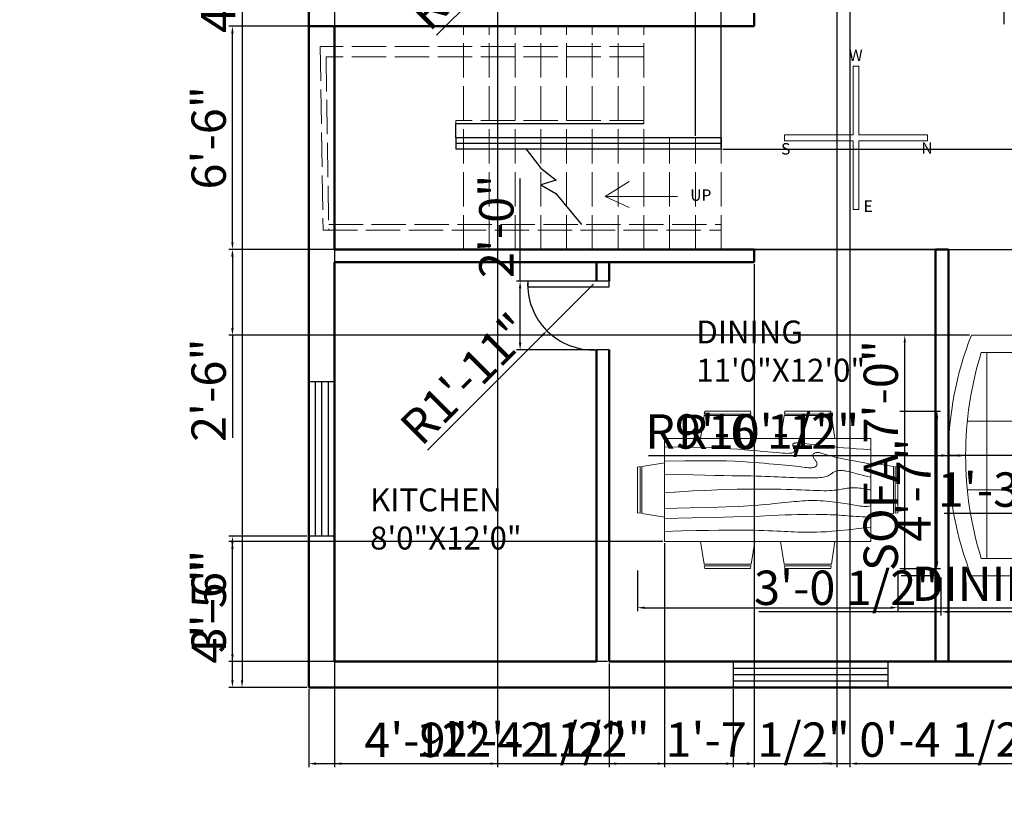
# Model space of a CAD drawing. Units: inches. Extents: x 2787 to 3354, y 1541 to 2259.
# Tile 1 of 3: x 2787 to 3131, y 1571 to 1842. Entities that reach past the tile are written whole.
import ezdxf

# ---------------------------------------------------------------- set-up
doc = ezdxf.new("R2010")
doc.units = ezdxf.units.IN
doc.linetypes.add('ACAD_ISO02W100', pattern=[15, 12, -3])
for name, color, linetype, lineweight in [('A-ANNO-DIMS', 2, 'Continuous', 18), ('A-ANNO-SYMB', 7, 'Continuous', 18), ('A-ANNO-TEXT', 7, 'Continuous', 18), ('A-AREA-IDEN', 7, 'Continuous', 25), ('A-DOOR', 4, 'Continuous', 25), ('A-FLOR-STRS', 7, 'Continuous', 25), ('A-FLOR-STRS-OVHD', 7, 'ACAD_ISO02W100', 18), ('A-FURN', 8, 'Continuous', 18), ('A-GLAZ', 4, 'Continuous', 25), ('A-WALL', 7, 'Continuous', 50)]:
    doc.layers.add(name, color=color, linetype=linetype, lineweight=lineweight)
doc.styles.get("Standard").update_dxf_attribs({"font": 'arial.ttf'})
doc.dimstyles.new('ISO-25', dxfattribs={"dimtxt": 12, "dimasz": 2.5, "dimexe": 1.25, "dimexo": 0.625, "dimtad": 1, "dimdec": 1, "dimlunit": 3, "dimtxsty": 'Standard', "dimcen": 2.5, "dimadec": 0, "dimazin": 0, "dimtfac": 1, "dimtdec": 1, "dimtmove": 0, "dimatfit": 3, "dimfxl": 1, "dimarcsym": 0})

# ---------------------------------------------------------------- blocks, each defined once
blk = doc.blocks.new('Window - Wood Frame 36 in. Wide plan')
for p, q in [((0, 6), (0, 0)), ((36, 6), (36, 0)), ((0, 4.5), (36, 4.5)), ((0, 3), (36, 3)), ((0, 1.5), (36, 1.5))]:
    blk.add_line(p, q)
blk = doc.blocks.new('Dining Set - 36 x 72 in.')
for p, q in [((-22.2343, 26.00059), (-23.4847, 17.99762)), ((-22.2304, 26), (-5.7608, 26)), ((-22, 27.5), (-22.1562, 26.50042)), ((-5.8416, 26.5), (-22.1534, 26.5)), ((-22, 27.5), (-6, 27.5)), ((-5.8437, 26.49966), (-6, 27.5)), ((-4.5152, 17.99762), (-5.7655, 25.99926)), ((5.7657, 26.00059), (4.5153, 17.99762)), ((5.7696, 26), (22.2392, 26)), ((6, 27.5), (5.8438, 26.50042)), ((22.1584, 26.5), (5.8466, 26.5)), ((6, 27.5), (22, 27.5)), ((22.1563, 26.49966), (22, 27.5)), ((23.4848, 17.99762), (22.2345, 25.99926)), ((36, 18), (-36, 18)), ((-36, 18), (-36, -18)), ((36, -18), (36, 18)), ((-45.5, 8), (-44.5004, 8.15617)), ((-45.5, 8), (-45.5, -8)), ((-44.5, -8.15843), (-44.5, 8.15338)), ((-44.0006, 8.23428), (-35.9976, 9.48474)), ((-44, 8.23041), (-44, -8.23915)), ((44.0006, 8.23428), (35.9976, 9.48474)), ((44, 8.23041), (44, -8.23915)), ((44.5, -8.15843), (44.5, 8.15338)), ((45.5, 8), (44.5005, 8.15617)), ((45.5, 8), (45.5, -8)), ((-44.4997, -8.15631), (-45.5, -8)), ((-35.9976, -9.48476), (-43.9993, -8.2345)), ((35.9976, -9.48476), (43.9993, -8.2345)), ((44.4997, -8.15631), (45.5, -8)), ((-36, -18), (36, -18)), ((-22.2343, -26.0006), (-23.4847, -17.99762)), ((-4.5152, -17.99762), (-5.7655, -25.99928)), ((5.7657, -26.0006), (4.5153, -17.99762)), ((23.4848, -17.99762), (22.2345, -25.99928)), ((-22.2304, -26), (-5.7608, -26)), ((-22, -27.5), (-22.1562, -26.50044)), ((-5.8416, -26.5), (-22.1534, -26.5)), ((-22, -27.5), (-6, -27.5)), ((-5.8437, -26.49967), (-6, -27.5)), ((5.7696, -26), (22.2392, -26)), ((6, -27.5), (5.8438, -26.50044)), ((22.1584, -26.5), (5.8466, -26.5)), ((6, -27.5), (22, -27.5)), ((22.1563, -26.49967), (22, -27.5))]:
    blk.add_line(p, q)
for points in [[(-36, 15), (-31.1772, 14.97754), (-26.8079, 14.91406), (-22.8538, 14.81543), (-19.276, 14.6875), (-16.0362, 14.53613), (-13.0957, 14.36718), (-10.4159, 14.18652), (-7.9583, 14), (-5.6904, 13.81315), (-3.6035, 13.63021), (-1.6954, 13.45508), (0.0365, 13.29166), (1.5945, 13.14388), (2.9811, 13.01562), (4.1988, 12.9108), (5.25, 12.83333), (6.1393, 12.78613), (6.8802, 12.76823), (7.4883, 12.77767), (7.9792, 12.8125), (8.3685, 12.87077), (8.6719, 12.95052), (8.9049, 13.0498), (9.0833, 13.16666), (9.2205, 13.29899), (9.3216, 13.44401), (9.3895, 13.59879), (9.4271, 13.76041), (9.4373, 13.92594), (9.4232, 14.09245), (9.3875, 14.257), (9.3333, 14.41666), (9.2638, 14.56917), (9.1836, 14.71484), (9.0975, 14.85465), (9.0104, 14.98958), (8.9272, 15.1206), (8.8529, 15.2487), (8.7922, 15.37483), (8.75, 15.5), (8.7305, 15.62467), (8.7344, 15.74739), (8.7617, 15.86621), (8.8125, 15.97916), (8.8867, 16.08431), (8.9844, 16.17968), (9.1055, 16.26334), (9.25, 16.33333), (9.4189, 16.38802), (9.6172, 16.42708), (9.8506, 16.45052), (10.125, 16.45833), (10.4463, 16.45052), (10.8203, 16.42708), (11.2529, 16.38802), (11.75, 16.33333), (12.3184, 16.26318), (12.9694, 16.17838), (13.7151, 16.07991), (14.5677, 15.96875), (15.5395, 15.84586), (16.6426, 15.71224), (17.8893, 15.56884), (19.2917, 15.41666), (20.859, 15.25667), (22.5879, 15.08984), (24.4721, 14.91715), (26.5052, 14.73958), (28.6809, 14.5581), (30.9929, 14.3737), (33.4347, 14.18733), (36, 14)], [(-36, 10), (-28.9766, 10.14274), (-23.1725, 10.20442), (-18.4241, 10.19775), (-14.5677, 10.13541), (-11.4399, 10.03011), (-8.877, 9.89453), (-6.7154, 9.74137), (-4.7917, 9.58333), (-2.9698, 9.43082), (-1.2246, 9.28515), (0.4415, 9.14534), (2.026, 9.01041), (3.5266, 8.87939), (4.9408, 8.7513), (6.266, 8.62516), (7.5, 8.5), (8.6411, 8.37549), (9.6914, 8.2539), (10.6538, 8.13818), (11.5312, 8.03125), (12.3267, 7.93603), (13.043, 7.85547), (13.6831, 7.79248), (14.25, 7.75), (14.7471, 7.7303), (15.1797, 7.73307), (15.5537, 7.75732), (15.875, 7.80208), (16.1494, 7.86637), (16.3828, 7.94922), (16.5811, 8.04964), (16.75, 8.16666), (16.8944, 8.29915), (17.0143, 8.44531), (17.1089, 8.60319), (17.1771, 8.77083), (17.218, 8.94629), (17.2305, 9.1276), (17.2137, 9.31282), (17.1667, 9.5), (17.0895, 9.6875), (16.987, 9.875), (16.8649, 10.0625), (16.7292, 10.25), (16.5856, 10.4375), (16.4401, 10.625), (16.2985, 10.8125), (16.1667, 11), (16.05, 11.18733), (15.9518, 11.3737), (15.8752, 11.5581), (15.8229, 11.73958), (15.798, 11.91715), (15.8034, 12.08984), (15.842, 12.25667), (15.9167, 12.41666), (16.0295, 12.56836), (16.1784, 12.70833), (16.3605, 12.83268), (16.5729, 12.9375), (16.8127, 13.01888), (17.0768, 13.07291), (17.3625, 13.0957), (17.6667, 13.08333), (17.9894, 13.03312), (18.3418, 12.94726), (18.7382, 12.82918), (19.1927, 12.68229), (19.7195, 12.51001), (20.3327, 12.31575), (21.0465, 12.10294), (21.875, 11.875), (22.8357, 11.63354), (23.959, 11.37304), (25.2786, 11.08618), (26.8282, 10.76562), (28.6414, 10.40405), (30.752, 9.99414), (33.1936, 9.52856), (36, 9)], [(-36, 5.5), (-30.7157, 5.3348), (-26.069, 5.20963), (-21.9946, 5.11767), (-18.4271, 5.05208), (-15.3009, 5.00602), (-12.5508, 4.97265), (-10.1112, 4.94515), (-7.9167, 4.91666), (-5.909, 4.88167), (-4.0586, 4.83984), (-2.3429, 4.79215), (-0.7396, 4.73958), (0.7739, 4.6831), (2.22, 4.6237), (3.6213, 4.56233), (5, 4.5), (6.373, 4.43782), (7.7344, 4.3776), (9.0723, 4.32129), (10.375, 4.27083), (11.6309, 4.22819), (12.8281, 4.19531), (13.9551, 4.17415), (15, 4.16666), (15.954, 4.17448), (16.819, 4.19791), (17.6001, 4.23698), (18.3021, 4.29166), (18.9299, 4.36198), (19.4883, 4.44791), (19.9823, 4.54948), (20.4167, 4.66666), (20.7969, 4.79899), (21.1302, 4.94401), (21.4245, 5.09879), (21.6875, 5.26041), (21.9271, 5.42594), (22.1511, 5.59245), (22.3672, 5.757), (22.5834, 5.91666), (22.8065, 6.06868), (23.0404, 6.21093), (23.2879, 6.34147), (23.5521, 6.45833), (23.8358, 6.55957), (24.142, 6.64323), (24.4735, 6.70735), (24.8334, 6.75), (25.2235, 6.76969), (25.642, 6.76692), (26.0858, 6.74267), (26.5521, 6.69791), (27.0379, 6.63362), (27.5404, 6.55078), (28.0565, 6.45036), (28.5834, 6.33333), (29.1242, 6.19987), (29.7071, 6.04687), (30.3661, 5.87044), (31.1354, 5.66666), (32.0493, 5.43164), (33.142, 5.16146), (34.4475, 4.85221), (36, 4.5)], [(-36, -1), (-30.7915, -0.6591), (-26.0195, -0.38216), (-21.6519, -0.16284), (-17.6563, 0.00521), (-14.0005, 0.12833), (-10.6523, 0.21289), (-7.5796, 0.26522), (-4.75, 0.29166), (-2.134, 0.29793), (0.2878, 0.28711), (2.5317, 0.26163), (4.6146, 0.22396), (6.5529, 0.17651), (8.3633, 0.12174), (10.0623, 0.06209), (11.6667, 0), (13.1899, -0.06201), (14.6341, -0.1211), (15.9982, -0.17432), (17.2813, -0.21875), (18.4823, -0.25147), (19.6003, -0.26953), (20.6343, -0.27002), (21.5834, -0.25), (22.4481, -0.20768), (23.2357, -0.14584), (23.9549, -0.06836), (24.6146, 0.02083), (25.2235, 0.11784), (25.7904, 0.21875), (26.3241, 0.31966), (26.8334, 0.41666), (27.3265, 0.50618), (27.8099, 0.58593), (28.2894, 0.65397), (28.7709, 0.70833), (29.2601, 0.74707), (29.763, 0.76823), (30.2855, 0.76985), (30.8334, 0.75), (31.4088, 0.70784), (31.9994, 0.64713), (32.589, 0.57275), (33.1615, 0.48958), (33.7008, 0.4025), (34.1908, 0.3164), (34.6153, 0.23616), (34.9584, 0.16666), (35.2099, 0.11165), (35.3848, 0.07031), (35.504, 0.04069), (35.5886, 0.02083), (35.6594, 0.00879), (35.7377, 0.0026), (35.8442, 0.00032), (36, 0)], [(-36, -6.5), (-27.1843, -6.31267), (-20.084, -6.1263), (-14.469, -5.9419), (-10.1094, -5.76042), (-6.7752, -5.58285), (-4.2363, -5.41016), (-2.2629, -5.24333), (-0.625, -5.08334), (0.8708, -4.93099), (2.2715, -4.78646), (3.5872, -4.64974), (4.8281, -4.52084), (6.0046, -4.39974), (7.127, -4.28646), (8.2053, -4.18099), (9.25, -4.08334), (10.2705, -3.99382), (11.2734, -3.91407), (12.2647, -3.84603), (13.25, -3.79167), (14.2354, -3.75293), (15.2266, -3.73177), (16.2295, -3.73015), (17.25, -3.75), (18.2912, -3.79248), (19.3451, -3.85547), (20.4009, -3.93604), (21.4479, -4.03125), (22.4754, -4.13819), (23.4727, -4.25391), (24.4289, -4.37549), (25.3334, -4.5), (26.1785, -4.62492), (26.9694, -4.74935), (27.7145, -4.87281), (28.4219, -4.99479), (29.1, -5.11483), (29.7572, -5.23242), (30.4016, -5.34709), (31.0417, -5.45834), (31.6837, -5.56437), (32.3262, -5.65821), (32.9658, -5.73153), (33.599, -5.77604), (34.2224, -5.78345), (34.8327, -5.74545), (35.4264, -5.65373), (36, -5.5)], [(-36, -10), (-26.4022, -9.81299), (-18.4675, -9.62891), (-11.9839, -9.45069), (-6.7396, -9.28125), (-2.5226, -9.12354), (0.8789, -8.98047), (3.6769, -8.85498), (6.0833, -8.75), (8.2767, -8.66765), (10.3021, -8.60677), (12.1712, -8.56543), (13.8958, -8.54167), (15.4876, -8.53353), (16.9583, -8.53907), (18.3197, -8.55632), (19.5834, -8.58334), (20.7616, -8.61841), (21.8685, -8.66081), (22.9188, -8.71004), (23.9271, -8.76563), (24.9081, -8.82707), (25.8763, -8.89388), (26.8465, -8.96558), (27.8334, -9.04167), (28.8474, -9.12118), (29.8828, -9.20117), (30.93, -9.27824), (31.9792, -9.34896), (33.0205, -9.40991), (34.0443, -9.45768), (35.0407, -9.48885), (36, -9.5)], [(-36, -14.5), (-30.0881, -14.33513), (-25.0332, -14.21224), (-20.7312, -14.12647), (-17.0781, -14.07292), (-13.97, -14.04671), (-11.3027, -14.04297), (-8.9724, -14.05681), (-6.875, -14.08334), (-4.9224, -14.11833), (-3.0905, -14.16016), (-1.3709, -14.20785), (0.2448, -14.26042), (1.7647, -14.3169), (3.1973, -14.3763), (4.5507, -14.43767), (5.8333, -14.5), (7.0554, -14.5621), (8.235, -14.62175), (9.3922, -14.67652), (10.5469, -14.72396), (11.7192, -14.76164), (12.929, -14.78711), (14.1965, -14.79794), (15.5417, -14.79167), (16.9933, -14.76424), (18.6152, -14.70508), (20.4804, -14.60197), (22.6615, -14.44271), (25.2312, -14.21509), (28.2624, -13.9069), (31.8277, -13.50594), (36, -13)]]:
    blk.add_lwpolyline(points)
blk = doc.blocks.new('*D6')
at = {"layer": 'A-ANNO-DIMS', "color": 0, "lineweight": -2, "transparency": 16777216}
for p, q in [((2887.4, 2088.26), (2863.48, 2088.26)), ((2864.73, 2085.76), (2864.73, 1610.76)), ((2887.4, 1608.26), (2863.48, 1608.26))]:
    blk.add_line(p, q, dxfattribs=at)
at = {"layer": 'A-ANNO-DIMS', "color": 0, "transparency": 16777216}
for points in [[(2864.31, 2085.76), (2865.14, 2085.76), (2864.73, 2088.26)], [(2864.31, 1610.76), (2865.14, 1610.76), (2864.73, 1608.26)]]:
    blk.add_solid(points, dxfattribs=at)
at = {"layer": 'Defpoints', "color": 0, "transparency": 16777216}
for p in [(2888.02, 2088.26), (2864.73, 1608.26), (2888.02, 1608.26)]:
    blk.add_point(p, dxfattribs=at)
at = {"layer": 'A-ANNO-DIMS', "color": 0, "transparency": 16777216, "insert": (2857.97, 1848.26), "char_height": 12, "attachment_point": 5, "rotation": 90}
blk.add_mtext("40'", dxfattribs=at)
blk = doc.blocks.new('Sofa - Roundback 7 ft.')
for p, q in [((-12.00002, -32.4421), (-12.00003, -6.5971)), ((11.99997, -32.4421), (11.99998, -6.5971)), ((-36.000027, -34), (-36.000027, -11.4696)), ((-35.999844, -13.3819), (35.9998, -13.3819)), ((35.99998, -34), (35.99998, -11.4696)), ((-36.000027, -32.4421), (35.99998, -32.4421))]:
    blk.add_line(p, q)
for points in [[(-36.000027, -34), (-42.000027, -34), (-42.000027, -8)], [(41.99998, -8), (41.99998, -34), (35.99998, -34)]]:
    blk.add_lwpolyline(points)
for centre, radius, start, end in [((0, -114.25), 114.25, 68.43141, 111.5686), ((-0.00001, -127.1968), 121.1968, 72.72033, 107.2797)]:
    blk.add_arc(centre, radius, start, end)
blk = doc.blocks.new('*D18')
at = {"layer": 'A-ANNO-DIMS', "color": 0, "lineweight": -2, "transparency": 16777216}
for p, q in [((2897.02, 1864.37), (2897.02, 1858.79)), ((2930.07, 1864.37), (2930.07, 1858.79)), ((2897.02, 1860.04), (2787.05, 1860.04)), ((2927.57, 1860.04), (2899.52, 1860.04))]:
    blk.add_line(p, q, dxfattribs=at)
at = {"layer": 'A-ANNO-DIMS', "color": 0, "transparency": 16777216}
for points in [[(2899.52, 1860.45), (2899.52, 1859.62), (2897.02, 1860.04)], [(2927.57, 1860.45), (2927.57, 1859.62), (2930.07, 1860.04)]]:
    blk.add_solid(points, dxfattribs=at)
at = {"layer": 'Defpoints', "color": 0, "transparency": 16777216}
for p in [(2897.02, 1864.99), (2930.07, 1864.99), (2897.02, 1860.04)]:
    blk.add_point(p, dxfattribs=at)
at = {"layer": 'A-ANNO-DIMS', "color": 0, "transparency": 16777216, "insert": (2840.79, 1866.87), "char_height": 12, "attachment_point": 5}
blk.add_mtext('WC 2\'-9" TYP.', dxfattribs=at)
blk = doc.blocks.new('*D24')
at = {"layer": 'A-ANNO-DIMS', "color": 0, "lineweight": -2, "transparency": 16777216}
for p, q in [((3002.87, 1649.12), (3002.87, 1634.84)), ((3093.87, 1649.12), (3093.87, 1634.84)), ((3005.37, 1636.09), (3091.37, 1636.09)), ((3093.87, 1636.09), (3229.51, 1636.09))]:
    blk.add_line(p, q, dxfattribs=at)
at = {"layer": 'A-ANNO-DIMS', "color": 0, "transparency": 16777216}
for points in [[(3005.37, 1636.51), (3005.37, 1635.68), (3002.87, 1636.09)], [(3091.37, 1636.51), (3091.37, 1635.68), (3093.87, 1636.09)]]:
    blk.add_solid(points, dxfattribs=at)
at = {"layer": 'Defpoints', "color": 0, "transparency": 16777216}
for p in [(3002.87, 1649.74), (3093.87, 1649.74), (3093.87, 1636.09)]:
    blk.add_point(p, dxfattribs=at)
at = {"layer": 'A-ANNO-DIMS', "color": 0, "transparency": 16777216, "insert": (3162.94, 1642.92), "char_height": 12, "attachment_point": 5}
blk.add_mtext('DINING SET 7\'-7"', dxfattribs=at)
blk = doc.blocks.new('*D25')
at = {"layer": 'A-ANNO-DIMS', "color": 0, "lineweight": -2, "transparency": 16777216}
for p, q in [((3094.49, 1704.74), (3108.77, 1704.74)), ((3107.52, 1652.24), (3107.52, 1702.24)), ((3094.49, 1649.74), (3108.77, 1649.74))]:
    blk.add_line(p, q, dxfattribs=at)
at = {"layer": 'A-ANNO-DIMS', "color": 0, "transparency": 16777216}
for points in [[(3107.1, 1702.24), (3107.94, 1702.24), (3107.52, 1704.74)], [(3107.1, 1652.24), (3107.94, 1652.24), (3107.52, 1649.74)]]:
    blk.add_solid(points, dxfattribs=at)
at = {"layer": 'Defpoints', "color": 0, "transparency": 16777216}
for p in [(3093.87, 1704.74), (3107.52, 1704.74), (3093.87, 1649.74)]:
    blk.add_point(p, dxfattribs=at)
at = {"layer": 'A-ANNO-DIMS', "color": 0, "transparency": 16777216, "insert": (3100.89, 1677.24), "char_height": 12, "attachment_point": 5, "rotation": 90}
blk.add_mtext('4\'-7"', dxfattribs=at)
blk = doc.blocks.new('*D26')
at = {"layer": 'A-ANNO-DIMS', "color": 0, "lineweight": -2, "transparency": 16777216}
for p, q in [((3108.23, 1731.26), (3095.01, 1731.26)), ((3096.26, 1649.76), (3096.26, 1728.76)), ((3108.23, 1647.26), (3095.01, 1647.26))]:
    blk.add_line(p, q, dxfattribs=at)
at = {"layer": 'A-ANNO-DIMS', "color": 0, "transparency": 16777216}
for points in [[(3095.84, 1728.76), (3096.67, 1728.76), (3096.26, 1731.26)], [(3095.84, 1649.76), (3096.67, 1649.76), (3096.26, 1647.26)]]:
    blk.add_solid(points, dxfattribs=at)
at = {"layer": 'Defpoints', "color": 0, "transparency": 16777216}
for p in [(3096.26, 1731.26), (3108.86, 1731.26), (3108.86, 1647.26)]:
    blk.add_point(p, dxfattribs=at)
at = {"layer": 'A-ANNO-DIMS', "color": 0, "transparency": 16777216, "insert": (3089.42, 1689.26), "char_height": 12, "attachment_point": 5, "rotation": 90}
blk.add_mtext('SOFA 7\'-0"', dxfattribs=at)
blk = doc.blocks.new('*D27')
at = {"layer": 'A-ANNO-DIMS', "color": 0, "lineweight": -2, "transparency": 16777216}
for p, q in [((3108.86, 1646.64), (3108.86, 1633.41)), ((3145.52, 1646.64), (3145.52, 1633.41)), ((3108.86, 1634.66), (3045.25, 1634.66)), ((3143.02, 1634.66), (3111.36, 1634.66))]:
    blk.add_line(p, q, dxfattribs=at)
at = {"layer": 'A-ANNO-DIMS', "color": 0, "transparency": 16777216}
for points in [[(3111.36, 1635.08), (3111.36, 1634.24), (3108.86, 1634.66)], [(3143.02, 1635.08), (3143.02, 1634.24), (3145.52, 1634.66)]]:
    blk.add_solid(points, dxfattribs=at)
at = {"layer": 'Defpoints', "color": 0, "transparency": 16777216}
for p in [(3108.86, 1647.26), (3145.52, 1647.26), (3108.86, 1634.66)]:
    blk.add_point(p, dxfattribs=at)
at = {"layer": 'A-ANNO-DIMS', "color": 0, "transparency": 16777216, "insert": (3075.81, 1641.49), "char_height": 12, "attachment_point": 5}
blk.add_mtext('3\'-0 1/2"', dxfattribs=at)
blk = doc.blocks.new('*D31')
at = {"layer": 'A-ANNO-DIMS', "color": 0, "lineweight": -2, "transparency": 16777216}
for p, q in [((3172.5, 1672.84), (3172.5, 1667.72)), ((3188, 1672.84), (3188, 1667.72)), ((3172.5, 1668.97), (3110.02, 1668.97)), ((3185.5, 1668.97), (3175, 1668.97))]:
    blk.add_line(p, q, dxfattribs=at)
at = {"layer": 'A-ANNO-DIMS', "color": 0, "transparency": 16777216}
for points in [[(3175, 1669.39), (3175, 1668.55), (3172.5, 1668.97)], [(3185.5, 1669.39), (3185.5, 1668.55), (3188, 1668.97)]]:
    blk.add_solid(points, dxfattribs=at)
at = {"layer": 'Defpoints', "color": 0, "transparency": 16777216}
for p in [(3172.5, 1673.47), (3188, 1673.47), (3172.5, 1668.97)]:
    blk.add_point(p, dxfattribs=at)
at = {"layer": 'A-ANNO-DIMS', "color": 0, "transparency": 16777216, "insert": (3140.01, 1675.8), "char_height": 12, "attachment_point": 5}
blk.add_mtext('1\'-3 1/2"', dxfattribs=at)
blk = doc.blocks.new('*D36')
at = {"layer": 'A-ANNO-DIMS', "color": 0, "lineweight": -2, "transparency": 16777216}
for p, q in [((2887.4, 1661.04), (2860.12, 1661.04)), ((2861.37, 1610.76), (2861.37, 1658.54)), ((2887.4, 1608.26), (2860.12, 1608.26))]:
    blk.add_line(p, q, dxfattribs=at)
at = {"layer": 'A-ANNO-DIMS', "color": 0, "transparency": 16777216}
for points in [[(2860.96, 1658.54), (2861.79, 1658.54), (2861.37, 1661.04)], [(2860.96, 1610.76), (2861.79, 1610.76), (2861.37, 1608.26)]]:
    blk.add_solid(points, dxfattribs=at)
at = {"layer": 'Defpoints', "color": 0, "transparency": 16777216}
for p in [(2861.37, 1661.04), (2888.02, 1661.04), (2888.02, 1608.26)]:
    blk.add_point(p, dxfattribs=at)
at = {"layer": 'A-ANNO-DIMS', "color": 0, "transparency": 16777216, "insert": (2854.65, 1634.65), "char_height": 12, "attachment_point": 5, "rotation": 90}
blk.add_mtext('4\'-5"', dxfattribs=at)
blk = doc.blocks.new('*D40')
at = {"layer": 'A-ANNO-DIMS', "color": 0, "lineweight": -2, "transparency": 16777216}
for p, q in [((2888.02, 1607.64), (2888.02, 1580.36)), ((3036.32, 1607.64), (3036.32, 1580.36)), ((2890.52, 1581.61), (3033.82, 1581.61))]:
    blk.add_line(p, q, dxfattribs=at)
at = {"layer": 'A-ANNO-DIMS', "color": 0, "transparency": 16777216}
for points in [[(2890.52, 1582.03), (2890.52, 1581.19), (2888.02, 1581.61)], [(3033.82, 1582.03), (3033.82, 1581.19), (3036.32, 1581.61)]]:
    blk.add_solid(points, dxfattribs=at)
at = {"layer": 'Defpoints', "color": 0, "transparency": 16777216}
for p in [(2888.02, 1608.26), (3036.32, 1608.26), (3036.32, 1581.61)]:
    blk.add_point(p, dxfattribs=at)
at = {"layer": 'A-ANNO-DIMS', "color": 0, "transparency": 16777216, "insert": (2962.17, 1588.44), "char_height": 12, "attachment_point": 5}
blk.add_mtext('12\'-4 1/2"', dxfattribs=at)
blk = doc.blocks.new('*D43')
at = {"layer": 'A-ANNO-DIMS', "color": 0, "lineweight": -2, "transparency": 16777216}
for p, q in [((2961.87, 1750.14), (2961.87, 1785.99)), ((2987.9, 1750.14), (2960.62, 1750.14)), ((2961.87, 1728.64), (2961.87, 1747.64)), ((2987.9, 1726.14), (2960.62, 1726.14))]:
    blk.add_line(p, q, dxfattribs=at)
at = {"layer": 'A-ANNO-DIMS', "color": 0, "transparency": 16777216}
for points in [[(2961.46, 1747.64), (2962.29, 1747.64), (2961.87, 1750.14)], [(2961.46, 1728.64), (2962.29, 1728.64), (2961.87, 1726.14)]]:
    blk.add_solid(points, dxfattribs=at)
at = {"layer": 'Defpoints', "color": 0, "transparency": 16777216}
for p in [(2961.87, 1750.14), (2988.52, 1750.14), (2988.52, 1726.14)]:
    blk.add_point(p, dxfattribs=at)
at = {"layer": 'A-ANNO-DIMS', "color": 0, "transparency": 16777216, "insert": (2955.12, 1769.31), "char_height": 12, "attachment_point": 5, "rotation": 90}
blk.add_mtext('2\'-0"', dxfattribs=at)
blk = doc.blocks.new('*D44')
at = {"layer": 'A-ANNO-DIMS', "color": 0, "lineweight": -2, "transparency": 16777216}
for p, q in [((2896.4, 1839.26), (2860.12, 1839.26)), ((2861.37, 1763.76), (2861.37, 1836.76)), ((2896.4, 1761.26), (2860.12, 1761.26))]:
    blk.add_line(p, q, dxfattribs=at)
at = {"layer": 'A-ANNO-DIMS', "color": 0, "transparency": 16777216}
for points in [[(2860.96, 1836.76), (2861.79, 1836.76), (2861.37, 1839.26)], [(2860.96, 1763.76), (2861.79, 1763.76), (2861.37, 1761.26)]]:
    blk.add_solid(points, dxfattribs=at)
at = {"layer": 'Defpoints', "color": 0, "transparency": 16777216}
for p in [(2861.37, 1839.26), (2897.02, 1839.26), (2897.02, 1761.26)]:
    blk.add_point(p, dxfattribs=at)
at = {"layer": 'A-ANNO-DIMS', "color": 0, "transparency": 16777216, "insert": (2854.62, 1800.26), "char_height": 12, "attachment_point": 5, "rotation": 90}
blk.add_mtext('6\'-6"', dxfattribs=at)
blk = doc.blocks.new('*D45')
at = {"layer": 'A-ANNO-DIMS', "color": 0, "lineweight": -2, "transparency": 16777216}
for p, q in [((2897.02, 1756.14), (2897.02, 1580.36)), ((3043.69, 1756.14), (3043.69, 1580.36)), ((2899.52, 1581.61), (3041.19, 1581.61))]:
    blk.add_line(p, q, dxfattribs=at)
at = {"layer": 'A-ANNO-DIMS', "color": 0, "transparency": 16777216}
for points in [[(2899.52, 1582.03), (2899.52, 1581.19), (2897.02, 1581.61)], [(3041.19, 1582.03), (3041.19, 1581.19), (3043.69, 1581.61)]]:
    blk.add_solid(points, dxfattribs=at)
at = {"layer": 'Defpoints', "color": 0, "transparency": 16777216}
for p in [(2897.02, 1756.76), (3043.69, 1756.76), (3043.69, 1581.61)]:
    blk.add_point(p, dxfattribs=at)
at = {"layer": 'A-ANNO-DIMS', "color": 0, "transparency": 16777216, "insert": (2970.36, 1588.44), "char_height": 12, "attachment_point": 5}
blk.add_mtext('12\'-2 1/2"', dxfattribs=at)
blk = doc.blocks.new('*D46')
at = {"layer": 'A-ANNO-DIMS', "color": 0, "lineweight": -2, "transparency": 16777216}
for p, q in [((3005.02, 1844.39), (3005.02, 2116.16)), ((3131.02, 1839.89), (3131.02, 2116.16)), ((3007.52, 2114.91), (3128.52, 2114.91))]:
    blk.add_line(p, q, dxfattribs=at)
at = {"layer": 'A-ANNO-DIMS', "color": 0, "transparency": 16777216}
for points in [[(3007.52, 2115.33), (3007.52, 2114.49), (3005.02, 2114.91)], [(3128.52, 2115.33), (3128.52, 2114.49), (3131.02, 2114.91)]]:
    blk.add_solid(points, dxfattribs=at)
at = {"layer": 'Defpoints', "color": 0, "transparency": 16777216}
for p in [(3131.02, 2114.91), (3005.02, 1843.76), (3131.02, 1839.26)]:
    blk.add_point(p, dxfattribs=at)
at = {"layer": 'A-ANNO-DIMS', "color": 0, "transparency": 16777216, "insert": (3068.02, 2121.66), "char_height": 12, "attachment_point": 5}
blk.add_mtext('10\'-6"', dxfattribs=at)
blk = doc.blocks.new('*D47')
at = {"layer": 'A-ANNO-DIMS', "color": 0, "lineweight": -2, "transparency": 16777216}
for p, q in [((3072.52, 2078.64), (3072.52, 1580.36)), ((3077.02, 2078.64), (3077.02, 1580.36)), ((3070.02, 1581.61), (3067.52, 1581.61)), ((3072.52, 1581.61), (3077.02, 1581.61)), ((3079.52, 1581.61), (3143.13, 1581.61))]:
    blk.add_line(p, q, dxfattribs=at)
at = {"layer": 'A-ANNO-DIMS', "color": 0, "transparency": 16777216}
for points in [[(3070.02, 1582.03), (3070.02, 1581.19), (3072.52, 1581.61)], [(3079.52, 1582.03), (3079.52, 1581.19), (3077.02, 1581.61)]]:
    blk.add_solid(points, dxfattribs=at)
at = {"layer": 'Defpoints', "color": 0, "transparency": 16777216}
for p in [(3072.52, 2079.26), (3077.02, 2079.26), (3077.02, 1581.61)]:
    blk.add_point(p, dxfattribs=at)
at = {"layer": 'A-ANNO-DIMS', "color": 0, "transparency": 16777216, "insert": (3112.58, 1588.44), "char_height": 12, "attachment_point": 5}
blk.add_mtext('0\'-4 1/2"', dxfattribs=at)
blk = doc.blocks.new('*D48')
at = {"layer": 'A-ANNO-DIMS', "color": 0, "lineweight": -2, "transparency": 16777216}
for p, q in [((3032.73, 1796.26), (3275.92, 1796.26)), ((3274.67, 1793.76), (3274.67, 1763.76)), ((3032.73, 1761.26), (3275.92, 1761.26)), ((3274.67, 1761.26), (3274.67, 1716.08))]:
    blk.add_line(p, q, dxfattribs=at)
at = {"layer": 'A-ANNO-DIMS', "color": 0, "transparency": 16777216}
for points in [[(3274.26, 1793.76), (3275.09, 1793.76), (3274.67, 1796.26)], [(3274.26, 1763.76), (3275.09, 1763.76), (3274.67, 1761.26)]]:
    blk.add_solid(points, dxfattribs=at)
at = {"layer": 'Defpoints', "color": 0, "transparency": 16777216}
for p in [(3032.1, 1796.26), (3032.1, 1761.26), (3274.67, 1761.26)]:
    blk.add_point(p, dxfattribs=at)
at = {"layer": 'A-ANNO-DIMS', "color": 0, "transparency": 16777216, "insert": (3268.02, 1737.42), "char_height": 12, "attachment_point": 5, "rotation": 90}
blk.add_mtext('2\'-11"', dxfattribs=at)
blk = doc.blocks.new('*D49')
at = {"layer": 'A-ANNO-DIMS', "color": 0, "lineweight": -2, "transparency": 16777216}
for p, q in [((3023.1, 1800.89), (3023.1, 2116.16)), ((3032.1, 1796.89), (3032.1, 2116.16)), ((3023.1, 2114.91), (2987.45, 2114.91)), ((3029.6, 2114.91), (3025.6, 2114.91))]:
    blk.add_line(p, q, dxfattribs=at)
at = {"layer": 'A-ANNO-DIMS', "color": 0, "transparency": 16777216}
for points in [[(3025.6, 2115.33), (3025.6, 2114.49), (3023.1, 2114.91)], [(3029.6, 2115.33), (3029.6, 2114.49), (3032.1, 2114.91)]]:
    blk.add_solid(points, dxfattribs=at)
at = {"layer": 'Defpoints', "color": 0, "transparency": 16777216}
for p in [(3023.1, 2114.91), (3023.1, 1800.26), (3032.1, 1796.26)]:
    blk.add_point(p, dxfattribs=at)
at = {"layer": 'A-ANNO-DIMS', "color": 0, "transparency": 16777216, "insert": (3004.03, 2121.66), "char_height": 12, "attachment_point": 5}
blk.add_mtext('0\'-9"', dxfattribs=at)
blk = doc.blocks.new('*D50')
at = {"layer": 'A-ANNO-DIMS', "color": 0, "lineweight": -2, "transparency": 16777216}
for p, q in [((2897.02, 2078.64), (2897.02, 1580.36)), ((2953.98, 2078.64), (2953.98, 1580.36)), ((2899.52, 1581.61), (2951.48, 1581.61))]:
    blk.add_line(p, q, dxfattribs=at)
at = {"layer": 'A-ANNO-DIMS', "color": 0, "transparency": 16777216}
for points in [[(2899.52, 1582.03), (2899.52, 1581.19), (2897.02, 1581.61)], [(2951.48, 1582.03), (2951.48, 1581.19), (2953.98, 1581.61)]]:
    blk.add_solid(points, dxfattribs=at)
at = {"layer": 'Defpoints', "color": 0, "transparency": 16777216}
for p in [(2897.02, 2079.26), (2953.98, 2079.26), (2953.98, 1581.61)]:
    blk.add_point(p, dxfattribs=at)
at = {"layer": 'A-ANNO-DIMS', "color": 0, "transparency": 16777216, "insert": (2925.5, 1588.36), "char_height": 12, "attachment_point": 5}
blk.add_mtext('4\'-9"', dxfattribs=at)
blk = doc.blocks.new('*D53')
at = {"layer": 'A-ANNO-DIMS', "color": 0, "lineweight": -2, "transparency": 16777216}
for p, q in [((3110.9, 1761.26), (2860.12, 1761.26)), ((2861.37, 1758.76), (2861.37, 1733.76)), ((3118.9, 1731.26), (2860.12, 1731.26)), ((2861.37, 1731.26), (2861.37, 1695.41))]:
    blk.add_line(p, q, dxfattribs=at)
at = {"layer": 'A-ANNO-DIMS', "color": 0, "transparency": 16777216}
for points in [[(2860.96, 1758.76), (2861.79, 1758.76), (2861.37, 1761.26)], [(2860.96, 1733.76), (2861.79, 1733.76), (2861.37, 1731.26)]]:
    blk.add_solid(points, dxfattribs=at)
at = {"layer": 'Defpoints', "color": 0, "transparency": 16777216}
for p in [(3111.52, 1761.26), (2861.37, 1731.26), (3119.52, 1731.26)]:
    blk.add_point(p, dxfattribs=at)
at = {"layer": 'A-ANNO-DIMS', "color": 0, "transparency": 16777216, "insert": (2854.62, 1712.08), "char_height": 12, "attachment_point": 5, "rotation": 90}
blk.add_mtext('2\'-6"', dxfattribs=at)
blk = doc.blocks.new('*D54')
at = {"layer": 'A-ANNO-DIMS', "color": 0, "lineweight": -2, "transparency": 16777216}
for p, q in [((3012.37, 1658.62), (3012.37, 1580.36)), ((2993.02, 1616.64), (2993.02, 1580.36)), ((2995.52, 1581.61), (3009.87, 1581.61)), ((3012.37, 1581.61), (3074.85, 1581.61))]:
    blk.add_line(p, q, dxfattribs=at)
at = {"layer": 'A-ANNO-DIMS', "color": 0, "transparency": 16777216}
for points in [[(2995.52, 1582.03), (2995.52, 1581.19), (2993.02, 1581.61)], [(3009.87, 1582.03), (3009.87, 1581.19), (3012.37, 1581.61)]]:
    blk.add_solid(points, dxfattribs=at)
at = {"layer": 'Defpoints', "color": 0, "transparency": 16777216}
for p in [(3012.37, 1659.24), (2993.02, 1617.26), (3012.37, 1581.61)]:
    blk.add_point(p, dxfattribs=at)
at = {"layer": 'A-ANNO-DIMS', "color": 0, "transparency": 16777216, "insert": (3044.86, 1588.44), "char_height": 12, "attachment_point": 5}
blk.add_mtext('1\'-7 1/2"', dxfattribs=at)
blk = doc.blocks.new('*D55')
at = {"layer": 'A-ANNO-DIMS', "color": 0, "lineweight": -2, "transparency": 16777216}
for p, q in [((3011.74, 1659.24), (2860.12, 1659.24)), ((2861.37, 1619.76), (2861.37, 1656.74)), ((2992.4, 1617.26), (2860.12, 1617.26))]:
    blk.add_line(p, q, dxfattribs=at)
at = {"layer": 'A-ANNO-DIMS', "color": 0, "transparency": 16777216}
for points in [[(2860.96, 1656.74), (2861.79, 1656.74), (2861.37, 1659.24)], [(2860.96, 1619.76), (2861.79, 1619.76), (2861.37, 1617.26)]]:
    blk.add_solid(points, dxfattribs=at)
at = {"layer": 'Defpoints', "color": 0, "transparency": 16777216}
for p in [(2861.37, 1659.24), (3012.37, 1659.24), (2993.02, 1617.26)]:
    blk.add_point(p, dxfattribs=at)
at = {"layer": 'A-ANNO-DIMS', "color": 0, "transparency": 16777216, "insert": (2854.62, 1638.25), "char_height": 12, "attachment_point": 5, "rotation": 90}
blk.add_mtext('3\'-6"', dxfattribs=at)
blk = doc.blocks.new('*D61')
at = {"layer": 'A-ANNO-DIMS', "color": 0, "lineweight": -2, "transparency": 16777216}
for p, q in [((2987.52, 1749.14), (2971.24, 1732.86)), ((2929.56, 1691.17), (2969.48, 1731.09))]:
    blk.add_line(p, q, dxfattribs=at)
at = {"layer": 'A-ANNO-DIMS', "color": 0, "transparency": 16777216}
blk.add_solid([(2969.18, 1731.38), (2969.77, 1730.8), (2971.24, 1732.86)], dxfattribs=at)
at = {"layer": 'Defpoints', "color": 0, "transparency": 16777216}
for p in [(2987.52, 1749.14), (2971.24, 1732.86)]:
    blk.add_point(p, dxfattribs=at)
at = {"layer": 'A-ANNO-DIMS', "color": 0, "transparency": 16777216, "insert": (2943.93, 1714.95), "char_height": 12, "attachment_point": 5, "rotation": 44.9993}
blk.add_mtext('R1\'-11"', dxfattribs=at)
blk = doc.blocks.new('*D62')
at = {"layer": 'A-ANNO-DIMS', "color": 0, "lineweight": -2, "transparency": 16777216}
for p, q in [((2999.77, 1903.18), (2987.57, 1890.97)), ((2932.7, 1836.1), (2985.8, 1889.21))]:
    blk.add_line(p, q, dxfattribs=at)
at = {"layer": 'A-ANNO-DIMS', "color": 0, "transparency": 16777216}
blk.add_solid([(2985.5, 1889.5), (2986.09, 1888.91), (2987.57, 1890.97)], dxfattribs=at)
at = {"layer": 'Defpoints', "color": 0, "transparency": 16777216}
for p in [(2999.77, 1903.18), (2987.57, 1890.97)]:
    blk.add_point(p, dxfattribs=at)
at = {"layer": 'A-ANNO-DIMS', "color": 0, "transparency": 16777216, "insert": (2953.53, 1866.6), "char_height": 12, "attachment_point": 5, "rotation": 45.0011}
blk.add_mtext('R1\'-5 1/2"', dxfattribs=at)
blk = doc.blocks.new('*D63')
at = {"layer": 'A-ANNO-DIMS', "color": 0, "lineweight": -2, "transparency": 16777216}
for p, q in [((3017.83, 1689.26), (3115.02, 1689.26)), ((3238.72, 1689.26), (3117.52, 1689.26))]:
    blk.add_line(p, q, dxfattribs=at)
at = {"layer": 'A-ANNO-DIMS', "color": 0, "transparency": 16777216}
blk.add_solid([(3115.02, 1689.68), (3115.02, 1688.84), (3117.52, 1689.26)], dxfattribs=at)
at = {"layer": 'Defpoints', "color": 0, "transparency": 16777216}
for p in [(3117.52, 1689.26), (3238.72, 1689.26)]:
    blk.add_point(p, dxfattribs=at)
at = {"layer": 'A-ANNO-DIMS', "color": 0, "transparency": 16777216, "insert": (3044.81, 1696.01), "char_height": 12, "attachment_point": 5}
blk.add_mtext('R10\'-1"', dxfattribs=at)
blk = doc.blocks.new('*D64')
at = {"layer": 'A-ANNO-DIMS', "color": 0, "lineweight": -2, "transparency": 16777216}
for p, q in [((3006.68, 1689.26), (3109.02, 1689.26)), ((3225.77, 1689.26), (3111.52, 1689.26))]:
    blk.add_line(p, q, dxfattribs=at)
at = {"layer": 'A-ANNO-DIMS', "color": 0, "transparency": 16777216}
blk.add_solid([(3109.02, 1689.68), (3109.02, 1688.84), (3111.52, 1689.26)], dxfattribs=at)
at = {"layer": 'Defpoints', "color": 0, "transparency": 16777216}
for p in [(3111.52, 1689.26), (3225.77, 1689.26)]:
    blk.add_point(p, dxfattribs=at)
at = {"layer": 'A-ANNO-DIMS', "color": 0, "transparency": 16777216, "insert": (3042.97, 1696.09), "char_height": 12, "attachment_point": 5}
blk.add_mtext('R9\'-6 1/2"', dxfattribs=at)

msp = doc.modelspace()

# ---------------------------------------------------------------- linework, layer by layer
at = {"layer": 'A-ANNO-SYMB'}
for p, q in [((3078.19, 1801.23), (3078.19, 1825.23)), ((3078.19, 1825.23), (3080.19, 1825.23)), ((3080.19, 1825.23), (3080.19, 1801.23)), ((3054.19, 1799.23), (3054.19, 1801.23)), ((3054.19, 1801.23), (3078.19, 1801.23)), ((3078.19, 1799.23), (3054.19, 1799.23)), ((3078.19, 1775.23), (3078.19, 1799.23)), ((3080.19, 1801.23), (3104.19, 1801.23)), ((3104.19, 1799.23), (3080.19, 1799.23)), ((3080.19, 1799.23), (3080.19, 1775.23)), ((3104.19, 1801.23), (3104.19, 1799.23)), ((2991.6, 1779.73), (2999.99, 1784.94)), ((3016.83, 1779.73), (2991.6, 1779.73)), ((2999.99, 1775.86), (2991.6, 1779.73)), ((3080.19, 1775.23), (3078.19, 1775.23)), ((3080.19, 1775.23), (3080.19, 1775.23))]:
    msp.add_line(p, q, dxfattribs=at)
at = {"layer": 'A-DOOR'}
for p, q in [((2988.52, 1750.14), (2964.52, 1750.14)), ((2964.52, 1750.14), (2964.52, 1748.14)), ((2964.52, 1748.14), (2993.02, 1748.14)), ((2993.02, 1750.14), (2988.52, 1750.14)), ((2993.02, 1748.14), (2993.02, 1750.14)), ((2993.02, 1726.14), (2988.52, 1726.14))]:
    msp.add_line(p, q, dxfattribs=at)
msp.add_arc((2987.52, 1749.14), 23.02, 177.5104, 272.4896, dxfattribs=at)
at = {"layer": 'A-FLOR-STRS'}
for p, q in [((2939.44, 1800.26), (2939.44, 1805.28)), ((2939.44, 1805.28), (3005.1, 1805.28)), ((3032.1, 1800.26), (2939.44, 1800.26)), ((2939.44, 1800.26), (2939.44, 1796.26)), ((3032.1, 1800.26), (3032.1, 1796.26)), ((3032.1, 1798.26), (2939.44, 1798.26)), ((3032.1, 1796.26), (2939.44, 1796.26)), ((2963.97, 1796.26), (2969.1, 1789.65)), ((2969.1, 1789.65), (2974.41, 1785.44)), ((2974.41, 1785.44), (2969.1, 1783.86)), ((2969.1, 1783.86), (2974.3, 1780.8)), ((2974.3, 1780.8), (2983.37, 1770.01))]:
    msp.add_line(p, q, dxfattribs=at)
at = {"layer": 'A-FLOR-STRS-OVHD'}
for p, q in [((2942.1, 1761.26), (2942.1, 1839.26)), ((2951.1, 1761.26), (2951.1, 1839.26)), ((2960.1, 1761.26), (2960.1, 1839.26)), ((2969.1, 1761.26), (2969.1, 1839.26)), ((2978.1, 1761.26), (2978.1, 1839.26)), ((2987.1, 1761.26), (2987.1, 1839.26)), ((2996.1, 1761.26), (2996.1, 1839.26)), ((3005.1, 1761.26), (3005.1, 1839.26)), ((3005.1, 1832.11), (2892.05, 1832.11)), ((2892.05, 1832.11), (2893.02, 1768.01)), ((3005.1, 1832.11), (2892.05, 1832.11)), ((2894.11, 1828.48), (2895.02, 1768.01)), ((3005.1, 1828.48), (2894.11, 1828.48)), ((3005.1, 1806.28), (2939.44, 1806.28)), ((2939.44, 1806.28), (2939.44, 1805.28)), ((3005.1, 1805.28), (3005.1, 1806.28)), ((3005.1, 1805.28), (3005.1, 1805.28)), ((3014.1, 1761.26), (3014.1, 1800.26)), ((3023.1, 1761.26), (3023.1, 1800.26)), ((3032.1, 1761.26), (3032.1, 1800.26)), ((3032.1, 1800.26), (3032.1, 1800.26)), ((2894.99, 1770.01), (3032.1, 1770.01)), ((2896.99, 1770.01), (2897.02, 1768.01)), ((2893.02, 1768.01), (3032.1, 1768.01))]:
    msp.add_line(p, q, dxfattribs=at)
at = {"layer": 'A-WALL'}
for p, q in [((2888.02, 1608.26), (2888.02, 2088.26)), ((3043.69, 1843.76), (3043.69, 1839.26)), ((2888.02, 1839.26), (3005.02, 1839.26)), ((2897.02, 1761.26), (2897.02, 1839.26)), ((3043.69, 1839.26), (3005.02, 1839.26)), ((3043.69, 1761.26), (2897.02, 1761.26)), ((3043.69, 1761.26), (3043.69, 1756.76)), ((3111.52, 1761.26), (3107.02, 1761.26)), ((3107.02, 1761.26), (3107.02, 1617.26)), ((3111.52, 1761.26), (3111.52, 1617.26)), ((2897.02, 1617.26), (2897.02, 1756.76)), ((2988.52, 1756.76), (2897.02, 1756.76)), ((2988.52, 1750.14), (2988.52, 1756.76)), ((3043.69, 1756.76), (2988.52, 1756.76)), ((2993.02, 1750.14), (2993.02, 1756.76)), ((2988.52, 1617.26), (2988.52, 1726.14)), ((2993.02, 1617.26), (2993.02, 1726.14)), ((2988.52, 1617.26), (2897.02, 1617.26)), ((3184.62, 1617.26), (2993.02, 1617.26)), ((3184.62, 1608.26), (2888.02, 1608.26))]:
    msp.add_line(p, q, dxfattribs=at)

# ---------------------------------------------------------------- block references
at = {"layer": 'A-FURN', "rotation": 90}
msp.add_blockref('Sofa - Roundback 7 ft.', (3111.52, 1689.26), dxfattribs=at)
at = {"layer": 'A-FURN'}
msp.add_blockref('Dining Set - 36 x 72 in.', (3048.37, 1677.24), dxfattribs=at)
at = {"layer": 'A-GLAZ', "xscale": 1.5, "yscale": 1.5, "zscale": 1.5, "rotation": 270}
msp.add_blockref('Window - Wood Frame 36 in. Wide plan', (2888.02, 1715.04), dxfattribs=at)
at = {"layer": 'A-GLAZ', "xscale": 1.5, "yscale": 1.5, "zscale": 1.5}
msp.add_blockref('Window - Wood Frame 36 in. Wide plan', (3036.32, 1608.26), dxfattribs=at)

# ---------------------------------------------------------------- texts
at = {"layer": 'A-ANNO-SYMB', "char_height": 4, "attachment_point": 1}
for s, insert in [('W', (3076.75, 1831.09)), ('S', (3053.03, 1798.39)), ('N', (3102.04, 1798.67)), ('E', (3081.85, 1778.36))]:
    msp.add_mtext(s, dxfattribs=dict(at, insert=insert))
at = {"layer": 'A-ANNO-TEXT', "insert": (3021.31, 1782.23), "char_height": 4, "attachment_point": 1}
msp.add_mtext('UP', dxfattribs=at)
at = {"layer": 'A-AREA-IDEN', "char_height": 8, "attachment_point": 1}
for s, insert in [('DINING\\P11\'0"X12\'0"', (3023.43, 1736.4)), ('KITCHEN\\P8\'0"X12\'0"', (2909.47, 1677.75))]:
    msp.add_mtext_dynamic_manual_height_columns(s, width=129.1776, gutter_width=12.5, heights=[0], dxfattribs=dict(at, insert=insert))

# ---------------------------------------------------------------- dimensions: what is measured, and where the dimension line sits
at = {"layer": 'A-ANNO-DIMS'}
for base, p1, p2, picture, middle in [((3023.1, 2114.91), (3032.1, 1796.26), (3023.1, 1800.26), '*D49', (3004.03, 2121.66)), ((3131.02, 2114.91), (3005.02, 1843.76), (3131.02, 1839.26), '*D46', (3068.02, 2121.66)), ((2953.98, 1581.61), (2897.02, 2079.26), (2953.98, 2079.26), '*D50', (2925.5, 1588.36)), ((3077.02, 1581.61), (3072.52, 2079.26), (3077.02, 2079.26), '*D47', (3112.58, 1588.44)), ((3043.69, 1581.61), (2897.02, 1756.76), (3043.69, 1756.76), '*D45', (2970.36, 1588.44)), ((3012.3699, 1581.611), (2993.024, 1617.261), (3012.3699, 1659.2425), '*D54', (3044.8605, 1588.4406)), ((3036.32, 1581.61), (2888.02, 1608.26), (3036.32, 1608.26), '*D40', (2962.17, 1588.44))]:
    dim = msp.add_linear_dim(base=base, p1=p1, p2=p2, dimstyle='ISO-25', override={"dimdec": 1, "dimlfac": 1, "dimrnd": 0, "dimzin": 1, "dimdsep": 46, "dimlunit": 4, "dimfrac": 2}, dxfattribs=at)
    dim.commit()
    dim.dimension.update_dxf_attribs({"geometry": picture, "text_midpoint": middle})
for base, p1, p2, angle, override, picture, middle in [((2864.73, 1608.26), (2888.02, 2088.26), (2888.02, 1608.26), 90, {"dimclrd": 0, "dimclre": 0, "dimclrt": 0}, '*D6', (2857.97, 1848.26)), ((2861.37, 1839.26), (2897.02, 1761.26), (2897.02, 1839.26), 90, {"dimdec": 1, "dimlfac": 1, "dimrnd": 0, "dimzin": 1, "dimdsep": 46, "dimlunit": 4, "dimfrac": 2}, '*D44', (2854.62, 1800.26)), ((3274.67, 1761.26), (3032.1, 1796.26), (3032.1, 1761.26), 90, {"dimdec": 1, "dimlfac": 1, "dimrnd": 0, "dimzin": 1, "dimdsep": 46, "dimlunit": 4, "dimfrac": 2}, '*D48', (3268.02, 1737.42)), ((2961.87, 1750.14), (2988.52, 1726.14), (2988.52, 1750.14), 90, {"dimdec": 1, "dimlfac": 1, "dimrnd": 0, "dimzin": 1, "dimdsep": 46, "dimlunit": 4, "dimfrac": 2}, '*D43', (2955.12, 1769.31)), ((2861.37, 1731.26), (3111.52, 1761.26), (3119.52, 1731.26), 90, {"dimdec": 1, "dimlfac": 1, "dimrnd": 0, "dimzin": 1, "dimdsep": 46, "dimlunit": 4, "dimfrac": 2}, '*D53', (2854.62, 1712.08)), ((3107.52, 1704.74), (3093.87, 1649.74), (3093.87, 1704.74), 90, {"dimdec": 1, "dimlfac": 1, "dimrnd": 0, "dimzin": 1, "dimdsep": 46, "dimlunit": 4, "dimfrac": 2}, '*D25', (3100.89, 1677.24)), ((3172.5, 1668.97), (3188, 1673.47), (3172.5, 1673.47), 180, {"dimdec": 1, "dimlfac": 1, "dimrnd": 0, "dimzin": 1, "dimdsep": 46, "dimlunit": 4, "dimfrac": 2}, '*D31', (3140.01, 1675.8)), ((2861.37, 1659.24), (2993.02, 1617.26), (3012.37, 1659.24), 90, {"dimdec": 1, "dimlfac": 1, "dimrnd": 0, "dimzin": 1, "dimdsep": 46, "dimlunit": 4, "dimfrac": 2}, '*D55', (2854.62, 1638.25)), ((2861.37, 1661.04), (2888.02, 1608.26), (2888.02, 1661.04), 90, {"dimdec": 1, "dimlfac": 1, "dimrnd": 0, "dimzin": 1, "dimdsep": 46, "dimlunit": 4, "dimfrac": 2}, '*D36', (2854.65, 1634.65)), ((3108.86, 1634.66), (3145.52, 1647.26), (3108.86, 1647.26), 180, {"dimdec": 1, "dimlfac": 1, "dimrnd": 0, "dimzin": 1, "dimdsep": 46, "dimlunit": 4, "dimfrac": 2}, '*D27', (3075.81, 1641.49))]:
    dim = msp.add_linear_dim(base=base, p1=p1, p2=p2, angle=angle, dimstyle='ISO-25', override=override, dxfattribs=at)
    dim.commit()
    dim.dimension.update_dxf_attribs({"geometry": picture, "text_midpoint": middle})
for center, mpoint, picture, middle in [((2999.77, 1903.18), (2987.57, 1890.97), '*D62', (2953.53, 1866.6)), ((2987.52, 1749.14), (2971.24, 1732.86), '*D61', (2943.93, 1714.95))]:
    dim = msp.add_radius_dim(center=center, mpoint=mpoint, dimstyle='ISO-25', override={"dimdec": 1, "dimlfac": 1, "dimrnd": 0, "dimzin": 1, "dimdsep": 46, "dimlunit": 4, "dimfrac": 2}, dxfattribs=at)
    dim.commit()
    dim.dimension.update_dxf_attribs({"geometry": picture, "text_midpoint": middle})
for base, p1, p2, angle, text, picture, middle in [((2897.024, 1860.038), (2930.0702, 1864.9949), (2897.024, 1864.9949), 180, 'WC <> TYP.', '*D18', (2840.7871, 1866.8676)), ((3096.26, 1731.26), (3108.86, 1647.26), (3108.86, 1731.26), 90, 'SOFA <>', '*D26', (3089.42, 1689.26))]:
    dim = msp.add_linear_dim(base=base, p1=p1, p2=p2, angle=angle, text=text, dimstyle='ISO-25', override={"dimdec": 1, "dimlfac": 1, "dimrnd": 0, "dimzin": 1, "dimdsep": 46, "dimlunit": 4, "dimfrac": 2}, dxfattribs=at)
    dim.commit()
    dim.dimension.update_dxf_attribs({"geometry": picture, "text_midpoint": middle})
for center, mpoint, picture, middle in [((3225.77398, 1689.260969), (3111.52398, 1689.261), '*D64', (3042.97398, 1689.261)), ((3238.72, 1689.26), (3117.52, 1689.26), '*D63', (3044.81, 1689.26))]:
    dim = msp.add_radius_dim(center=center, mpoint=mpoint, dimstyle='ISO-25', override={"dimdec": 1, "dimlfac": 1, "dimrnd": 0, "dimzin": 1, "dimdsep": 46, "dimlunit": 4, "dimfrac": 2}, dxfattribs=at)
    dim.commit()
    dim.dimension.update_dxf_attribs({"geometry": picture, "text_midpoint": middle, "dimtype": 164})
dim = msp.add_linear_dim(base=(3093.87, 1636.09), p1=(3002.87, 1649.74), p2=(3093.87, 1649.74), text='DINING SET <>', dimstyle='ISO-25', override={"dimdec": 1, "dimlfac": 1, "dimrnd": 0, "dimzin": 1, "dimdsep": 46, "dimlunit": 4, "dimfrac": 2}, dxfattribs=at)
dim.commit()
dim.dimension.update_dxf_attribs({"geometry": '*D24', "text_midpoint": (3162.94, 1642.92)})

doc.saveas('drawing.dxf')
